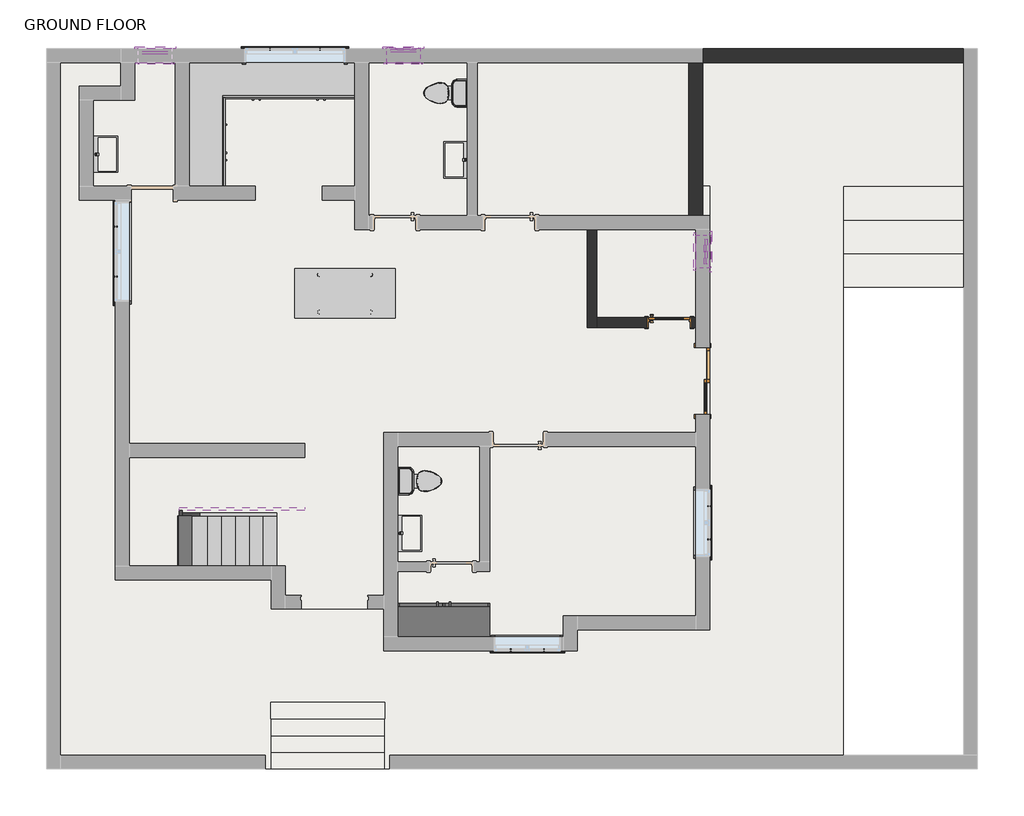
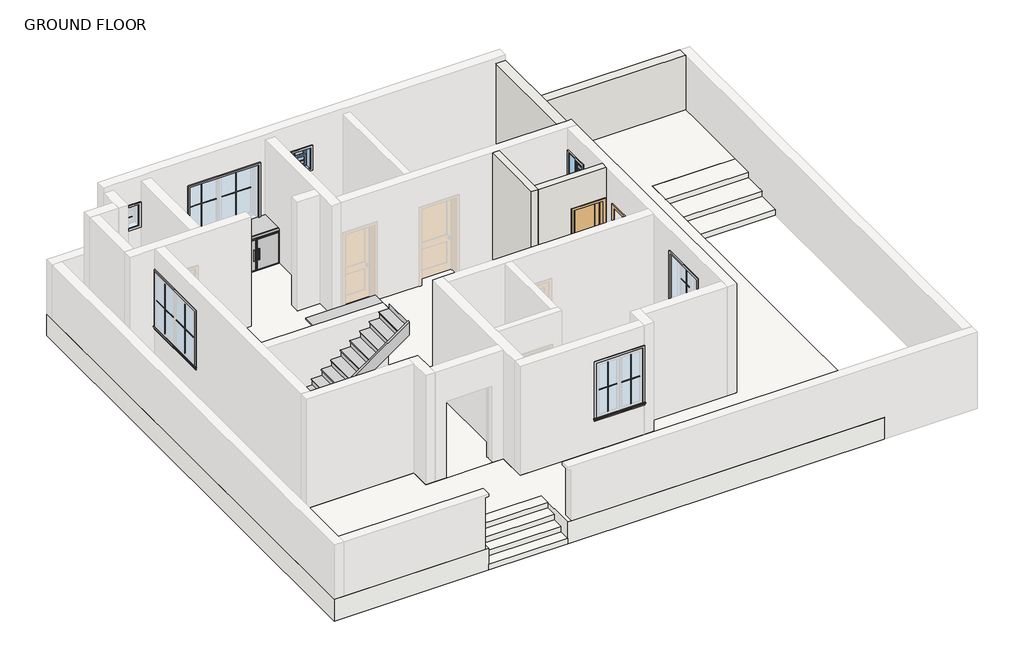
# One storey, part 2 of 2: 30 proxies, 9 slabs, 5 flow terminals, 4 walls, 3 members, 2 doors, 2 windows, 1 furniture element, 1 stair flight.
"""IFC4 building model written with IfcOpenShell, lengths in millimetres."""

from ifc_helpers import new_model, si_unit, frame, origin, origin_with_axes, place, context, project, spatial, polyline, outline, extrude, faceted_brep, transform, mapped, element, save
from components import generic_models_1_generic_models_1_c6f2978c, generic_models_2_generic_models_2_74e35ba5, muntin_pattern_2x2_muntin_pattern_2x2_e751b040, muntin_pattern_2x2_muntin_pattern_2x2_9cc8fee8, muntin_pattern_2x2_muntin_pattern_2x2_6dad3731, muntin_pattern_2x2_muntin_pattern_2x2_a30a3345, muntin_pattern_2x2_muntin_pattern_2x2_cfeb24ad, trim_window_exterior_flat_with_sill_c22f0c79, trim_window_exterior_flat_with_sill_92b9b949, trim_window_exterior_flat_with_sill_858dc10d, trim_window_interior_flat_picture_frame_d1f4d6ef, trim_window_interior_flat_picture_frame_3bb882cf, trim_window_interior_flat_picture_frame_3927330c, door_ae87caab, door_ff2e0a99, toilet_domestic_3d_toilet_domestic_3d_ba6479b0, toilet_domestic_3d_toilet_domestic_3d_30431060, sink_1_0003_sink_1_0003_9aba45dc, new_table_new_table_faa1bdb5, stair_flight_30e1afdc, window_double_hung_2_d0105baa

model = new_model("IFC4")

# Units and contexts
model_context = context("Model", 3, world=origin())
ifc_project = project(units=[si_unit("LENGTHUNIT", "METRE", prefix="MILLI")], contexts=[model_context])

# Site, building, storey
site = spatial("IfcSite", under=ifc_project)
building = spatial("IfcBuilding", under=site)
storey = spatial("IfcBuildingStorey", under=building, Name="GROUND FLOOR", Elevation=0.0)

# Proxies
placement = place(None, origin())
generic_models_1_generic_models_1_shape = generic_models_1_generic_models_1_c6f2978c(model_context)
element("IfcBuildingElementProxy", 1, Name="Generic Models 1 : Generic Models 1", ObjectType="Generic Models 1 : Generic Models 1", at=placement, inside=storey, context=model_context, shape_type="MappedRepresentation", body=[
    mapped(generic_models_1_generic_models_1_shape, transform((0.0, 0.0, 0.0), x_axis=(1.0, 0.0, 0.0), y_axis=(0.0, 1.0, 0.0), z_axis=(0.0, 0.0, 1.0))),
])
generic_models_2_generic_models_2_shape = generic_models_2_generic_models_2_74e35ba5(model_context)
element("IfcBuildingElementProxy", 2, Name="Generic Models 2 : Generic Models 2", ObjectType="Generic Models 2 : Generic Models 2", at=placement, inside=storey, context=model_context, shape_type="MappedRepresentation", body=[
    mapped(generic_models_2_generic_models_2_shape, transform((0.0, 0.0, 0.0), x_axis=(1.0, 0.0, 0.0), y_axis=(0.0, 1.0, 0.0), z_axis=(0.0, 0.0, 1.0))),
])
muntin_pattern_2x2_muntin_pattern_2x2_shape = muntin_pattern_2x2_muntin_pattern_2x2_e751b040(model_context)
element("IfcBuildingElementProxy", 3, Name="Muntin Pattern_2x2 : Muntin Pattern_2x2", ObjectType="Muntin Pattern_2x2 : Muntin Pattern_2x2", at=placement, inside=storey, context=model_context, shape_type="MappedRepresentation", body=[
    mapped(muntin_pattern_2x2_muntin_pattern_2x2_shape, transform((-8676.6951068, 1938.7752014, 984.25), x_axis=(0.0, 1.0, 0.0), y_axis=(-1.0, 0.0, 0.0), z_axis=(0.0, 0.0, 1.0))),
])
element("IfcBuildingElementProxy", 4, Name="Muntin Pattern_2x2 : Muntin Pattern_2x2", ObjectType="Muntin Pattern_2x2 : Muntin Pattern_2x2", at=placement, inside=storey, context=model_context, shape_type="MappedRepresentation", body=[
    mapped(muntin_pattern_2x2_muntin_pattern_2x2_shape, transform((-5865.2326068, 6093.2627014, 984.25), x_axis=(1.0, 0.0, 0.0), y_axis=(0.0, 1.0, 0.0), z_axis=(0.0, 0.0, 1.0))),
])
muntin_pattern_2x2_muntin_pattern_2x2_2_shape = muntin_pattern_2x2_muntin_pattern_2x2_9cc8fee8(model_context)
element("IfcBuildingElementProxy", 5, Name="Muntin Pattern_2x2 : Muntin Pattern_2x2", ObjectType="Muntin Pattern_2x2 : Muntin Pattern_2x2", at=placement, inside=storey, context=model_context, shape_type="MappedRepresentation", body=[
    mapped(muntin_pattern_2x2_muntin_pattern_2x2_2_shape, transform((-8676.6951068, 2850.0002014, 984.25), x_axis=(0.0, -1.0, 0.0), y_axis=(1.0, 0.0, 0.0), z_axis=(0.0, 0.0, 1.0))),
])
element("IfcBuildingElementProxy", 6, Name="Muntin Pattern_2x2 : Muntin Pattern_2x2", ObjectType="Muntin Pattern_2x2 : Muntin Pattern_2x2", at=placement, inside=storey, context=model_context, shape_type="MappedRepresentation", body=[
    mapped(muntin_pattern_2x2_muntin_pattern_2x2_2_shape, transform((-4954.0076068, 6093.2627014, 984.25), x_axis=(-1.0, 0.0, 0.0), y_axis=(0.0, -1.0, 0.0), z_axis=(0.0, 0.0, 1.0))),
])
muntin_pattern_2x2_muntin_pattern_2x2_3_shape = muntin_pattern_2x2_muntin_pattern_2x2_6dad3731(model_context)
element("IfcBuildingElementProxy", 7, Name="Muntin Pattern_2x2 : Muntin Pattern_2x2", ObjectType="Muntin Pattern_2x2 : Muntin Pattern_2x2", at=placement, inside=storey, context=model_context, shape_type="MappedRepresentation", body=[
    mapped(muntin_pattern_2x2_muntin_pattern_2x2_3_shape, transform((-864.6076068, -4885.8872986, 984.25), x_axis=(-1.0, 0.0, 0.0), y_axis=(0.0, -1.0, 0.0), z_axis=(0.0, 0.0, 1.0))),
])
element("IfcBuildingElementProxy", 8, Name="Muntin Pattern_2x2 : Muntin Pattern_2x2", ObjectType="Muntin Pattern_2x2 : Muntin Pattern_2x2", at=placement, inside=storey, context=model_context, shape_type="MappedRepresentation", body=[
    mapped(muntin_pattern_2x2_muntin_pattern_2x2_3_shape, transform((2150.0548932, -2255.3997986, 984.25), x_axis=(0.0, -1.0, 0.0), y_axis=(1.0, 0.0, 0.0), z_axis=(0.0, 0.0, 1.0))),
])
muntin_pattern_2x2_muntin_pattern_2x2_4_shape = muntin_pattern_2x2_muntin_pattern_2x2_a30a3345(model_context)
element("IfcBuildingElementProxy", 9, Name="Muntin Pattern_2x2 : Muntin Pattern_2x2", ObjectType="Muntin Pattern_2x2 : Muntin Pattern_2x2", at=placement, inside=storey, context=model_context, shape_type="MappedRepresentation", body=[
    mapped(muntin_pattern_2x2_muntin_pattern_2x2_4_shape, transform((-1471.0326068, -4885.8872986, 984.25), x_axis=(1.0, 0.0, 0.0), y_axis=(0.0, 1.0, 0.0), z_axis=(0.0, 0.0, 1.0))),
])
element("IfcBuildingElementProxy", 10, Name="Muntin Pattern_2x2 : Muntin Pattern_2x2", ObjectType="Muntin Pattern_2x2 : Muntin Pattern_2x2", at=placement, inside=storey, context=model_context, shape_type="MappedRepresentation", body=[
    mapped(muntin_pattern_2x2_muntin_pattern_2x2_4_shape, transform((2150.0548932, -2861.8247986, 984.25), x_axis=(0.0, 1.0, 0.0), y_axis=(-1.0, 0.0, 0.0), z_axis=(0.0, 0.0, 1.0))),
])
muntin_pattern_2x2_muntin_pattern_2x2_5_shape = muntin_pattern_2x2_muntin_pattern_2x2_cfeb24ad(model_context)
element("IfcBuildingElementProxy", 11, Name="Muntin Pattern_2x2 : Muntin Pattern_2x2", ObjectType="Muntin Pattern_2x2 : Muntin Pattern_2x2", at=placement, inside=storey, context=model_context, shape_type="MappedRepresentation", body=[
    mapped(muntin_pattern_2x2_muntin_pattern_2x2_5_shape, transform((2124.6548932, 2394.3877014, 2155.825), x_axis=(0.0, -1.0, 0.0), y_axis=(1.0, 0.0, 0.0), z_axis=(0.0, 0.0, 1.0))),
])
element("IfcBuildingElementProxy", 12, Name="Muntin Pattern_2x2 : Muntin Pattern_2x2", ObjectType="Muntin Pattern_2x2 : Muntin Pattern_2x2", at=placement, inside=storey, context=model_context, shape_type="MappedRepresentation", body=[
    mapped(muntin_pattern_2x2_muntin_pattern_2x2_5_shape, transform((2080.2048932, 2394.3877014, 1905.0), x_axis=(0.0, -1.0, 0.0), y_axis=(1.0, 0.0, 0.0), z_axis=(0.0, 0.0, 1.0))),
])
element("IfcBuildingElementProxy", 13, Name="Muntin Pattern_2x2 : Muntin Pattern_2x2", ObjectType="Muntin Pattern_2x2 : Muntin Pattern_2x2", at=placement, inside=storey, context=model_context, shape_type="MappedRepresentation", body=[
    mapped(muntin_pattern_2x2_muntin_pattern_2x2_5_shape, transform((-3428.4201068, 6067.8627014, 2155.825), x_axis=(1.0, 0.0, 0.0), y_axis=(0.0, 1.0, 0.0), z_axis=(0.0, 0.0, 1.0))),
])
element("IfcBuildingElementProxy", 14, Name="Muntin Pattern_2x2 : Muntin Pattern_2x2", ObjectType="Muntin Pattern_2x2 : Muntin Pattern_2x2", at=placement, inside=storey, context=model_context, shape_type="MappedRepresentation", body=[
    mapped(muntin_pattern_2x2_muntin_pattern_2x2_5_shape, transform((-3428.4201068, 6023.4127014, 1905.0), x_axis=(1.0, 0.0, 0.0), y_axis=(0.0, 1.0, 0.0), z_axis=(0.0, 0.0, 1.0))),
])
element("IfcBuildingElementProxy", 15, Name="Muntin Pattern_2x2 : Muntin Pattern_2x2", ObjectType="Muntin Pattern_2x2 : Muntin Pattern_2x2", at=placement, inside=storey, context=model_context, shape_type="MappedRepresentation", body=[
    mapped(muntin_pattern_2x2_muntin_pattern_2x2_5_shape, transform((-7962.3201068, 6067.8627014, 2155.825), x_axis=(1.0, 0.0, 0.0), y_axis=(0.0, 1.0, 0.0), z_axis=(0.0, 0.0, 1.0))),
])
element("IfcBuildingElementProxy", 16, Name="Muntin Pattern_2x2 : Muntin Pattern_2x2", ObjectType="Muntin Pattern_2x2 : Muntin Pattern_2x2", at=placement, inside=storey, context=model_context, shape_type="MappedRepresentation", body=[
    mapped(muntin_pattern_2x2_muntin_pattern_2x2_5_shape, transform((-7962.3201068, 6023.4127014, 1905.0), x_axis=(1.0, 0.0, 0.0), y_axis=(0.0, 1.0, 0.0), z_axis=(0.0, 0.0, 1.0))),
])
trim_window_exterior_flat_with_sill_shape = trim_window_exterior_flat_with_sill_c22f0c79(model_context)
element("IfcBuildingElementProxy", 17, Name="Trim-Window-Exterior-Flat : with Sill", ObjectType="Trim-Window-Exterior-Flat : with Sill", at=placement, inside=storey, context=model_context, shape_type="MappedRepresentation", body=[
    mapped(trim_window_exterior_flat_with_sill_shape, transform((-8686.2201068, 2394.3877014, 2438.4), x_axis=(0.0, -1.0, 0.0), y_axis=(0.0, 0.0, 1.0), z_axis=(-1.0, 0.0, 0.0))),
])
element("IfcBuildingElementProxy", 18, Name="Trim-Window-Exterior-Flat : with Sill", ObjectType="Trim-Window-Exterior-Flat : with Sill", at=placement, inside=storey, context=model_context, shape_type="MappedRepresentation", body=[
    mapped(trim_window_exterior_flat_with_sill_shape, transform((-5409.6201068, 6102.7877014, 2438.4), x_axis=(-1.0, 0.0, 0.0), y_axis=(0.0, 0.0, 1.0), z_axis=(0.0, 1.0, 0.0))),
])
trim_window_exterior_flat_with_sill_2_shape = trim_window_exterior_flat_with_sill_92b9b949(model_context)
element("IfcBuildingElementProxy", 19, Name="Trim-Window-Exterior-Flat : with Sill", ObjectType="Trim-Window-Exterior-Flat : with Sill", at=placement, inside=storey, context=model_context, shape_type="MappedRepresentation", body=[
    mapped(trim_window_exterior_flat_with_sill_2_shape, transform((-1167.8201068, -4895.4122986, 2438.4), x_axis=(1.0, 0.0, 0.0), y_axis=(0.0, 0.0, 1.0), z_axis=(0.0, -1.0, 0.0))),
])
element("IfcBuildingElementProxy", 20, Name="Trim-Window-Exterior-Flat : with Sill", ObjectType="Trim-Window-Exterior-Flat : with Sill", at=placement, inside=storey, context=model_context, shape_type="MappedRepresentation", body=[
    mapped(trim_window_exterior_flat_with_sill_2_shape, transform((2159.5798932, -2558.6122986, 2438.4), x_axis=(0.0, 1.0, 0.0), y_axis=(0.0, 0.0, 1.0), z_axis=(1.0, 0.0, 0.0))),
])
trim_window_exterior_flat_with_sill_3_shape = trim_window_exterior_flat_with_sill_858dc10d(model_context)
element("IfcBuildingElementProxy", 21, Name="Trim-Window-Exterior-Flat : with Sill", ObjectType="Trim-Window-Exterior-Flat : with Sill", at=placement, inside=storey, context=model_context, shape_type="MappedRepresentation", body=[
    mapped(trim_window_exterior_flat_with_sill_3_shape, transform((2159.5798932, 2394.3877014, 2438.4), x_axis=(0.0, 1.0, 0.0), y_axis=(0.0, 0.0, 1.0), z_axis=(1.0, 0.0, 0.0))),
])
element("IfcBuildingElementProxy", 22, Name="Trim-Window-Exterior-Flat : with Sill", ObjectType="Trim-Window-Exterior-Flat : with Sill", at=placement, inside=storey, context=model_context, shape_type="MappedRepresentation", body=[
    mapped(trim_window_exterior_flat_with_sill_3_shape, transform((-3428.4201068, 6102.7877014, 2438.4), x_axis=(-1.0, 0.0, 0.0), y_axis=(0.0, 0.0, 1.0), z_axis=(0.0, 1.0, 0.0))),
])
element("IfcBuildingElementProxy", 23, Name="Trim-Window-Exterior-Flat : with Sill", ObjectType="Trim-Window-Exterior-Flat : with Sill", at=placement, inside=storey, context=model_context, shape_type="MappedRepresentation", body=[
    mapped(trim_window_exterior_flat_with_sill_3_shape, transform((-7962.3201068, 6102.7877014, 2438.4), x_axis=(-1.0, 0.0, 0.0), y_axis=(0.0, 0.0, 1.0), z_axis=(0.0, 1.0, 0.0))),
])
trim_window_interior_flat_picture_frame_shape = trim_window_interior_flat_picture_frame_d1f4d6ef(model_context)
element("IfcBuildingElementProxy", 24, Name="Trim-Window-Interior-Flat : Picture Frame", ObjectType="Trim-Window-Interior-Flat : Picture Frame", at=placement, inside=storey, context=model_context, shape_type="MappedRepresentation", body=[
    mapped(trim_window_interior_flat_picture_frame_shape, transform((-8432.2201068, 2394.3877014, 2438.4), x_axis=(0.0, 1.0, 0.0), y_axis=(0.0, 0.0, 1.0), z_axis=(1.0, 0.0, 0.0))),
])
element("IfcBuildingElementProxy", 25, Name="Trim-Window-Interior-Flat : Picture Frame", ObjectType="Trim-Window-Interior-Flat : Picture Frame", at=placement, inside=storey, context=model_context, shape_type="MappedRepresentation", body=[
    mapped(trim_window_interior_flat_picture_frame_shape, transform((-5409.6201068, 5848.7877014, 2438.4), x_axis=(1.0, 0.0, 0.0), y_axis=(0.0, 0.0, 1.0), z_axis=(0.0, -1.0, 0.0))),
])
trim_window_interior_flat_picture_frame_2_shape = trim_window_interior_flat_picture_frame_3bb882cf(model_context)
element("IfcBuildingElementProxy", 26, Name="Trim-Window-Interior-Flat : Picture Frame", ObjectType="Trim-Window-Interior-Flat : Picture Frame", at=placement, inside=storey, context=model_context, shape_type="MappedRepresentation", body=[
    mapped(trim_window_interior_flat_picture_frame_2_shape, transform((-1167.8201068, -4641.4122986, 2438.4), x_axis=(-1.0, 0.0, 0.0), y_axis=(0.0, 0.0, 1.0), z_axis=(0.0, 1.0, 0.0))),
])
element("IfcBuildingElementProxy", 27, Name="Trim-Window-Interior-Flat : Picture Frame", ObjectType="Trim-Window-Interior-Flat : Picture Frame", at=placement, inside=storey, context=model_context, shape_type="MappedRepresentation", body=[
    mapped(trim_window_interior_flat_picture_frame_2_shape, transform((1905.5798932, -2558.6122986, 2438.4), x_axis=(0.0, -1.0, 0.0), y_axis=(0.0, 0.0, 1.0), z_axis=(-1.0, 0.0, 0.0))),
])
trim_window_interior_flat_picture_frame_3_shape = trim_window_interior_flat_picture_frame_3927330c(model_context)
element("IfcBuildingElementProxy", 28, Name="Trim-Window-Interior-Flat : Picture Frame", ObjectType="Trim-Window-Interior-Flat : Picture Frame", at=placement, inside=storey, context=model_context, shape_type="MappedRepresentation", body=[
    mapped(trim_window_interior_flat_picture_frame_3_shape, transform((1905.5798932, 2394.3877014, 2438.4), x_axis=(0.0, -1.0, 0.0), y_axis=(0.0, 0.0, 1.0), z_axis=(-1.0, 0.0, 0.0))),
])
element("IfcBuildingElementProxy", 29, Name="Trim-Window-Interior-Flat : Picture Frame", ObjectType="Trim-Window-Interior-Flat : Picture Frame", at=placement, inside=storey, context=model_context, shape_type="MappedRepresentation", body=[
    mapped(trim_window_interior_flat_picture_frame_3_shape, transform((-3428.4201068, 5848.7877014, 2438.4), x_axis=(1.0, 0.0, 0.0), y_axis=(0.0, 0.0, 1.0), z_axis=(0.0, -1.0, 0.0))),
])
element("IfcBuildingElementProxy", 30, Name="Trim-Window-Interior-Flat : Picture Frame", ObjectType="Trim-Window-Interior-Flat : Picture Frame", at=placement, inside=storey, context=model_context, shape_type="MappedRepresentation", body=[
    mapped(trim_window_interior_flat_picture_frame_3_shape, transform((-7962.3201068, 5848.7877014, 2438.4), x_axis=(1.0, 0.0, 0.0), y_axis=(0.0, 0.0, 1.0), z_axis=(0.0, -1.0, 0.0))),
])

# Doors
door_shape = door_ae87caab(model_context)
element("IfcDoor", 31, ObjectType="Door-Double-Sliding : 48\" x 84\"", at=placement, inside=storey, context=model_context, shape_type="MappedRepresentation", body=[
    mapped(door_shape, transform((1905.5798932, 32.1877014, 0.0), x_axis=(0.0, -1.0, 0.0), y_axis=(1.0, 0.0, 0.0), z_axis=(0.0, 0.0, 1.0))),
])
door_2_shape = door_ff2e0a99(model_context)
element("IfcDoor", 32, ObjectType="Door-Interior-Single-2_Panel-Wood : 2'6\"", at=placement, inside=storey, context=model_context, shape_type="MappedRepresentation", body=[
    mapped(door_2_shape, transform((1422.9798932, 1102.1627014, 0.0), x_axis=(1.0, 0.0, 0.0), y_axis=(0.0, 1.0, 0.0), z_axis=(0.0, 0.0, 1.0))),
])

# Flow terminals
toilet_domestic_3d_toilet_domestic_3d_shape = toilet_domestic_3d_toilet_domestic_3d_ba6479b0(model_context)
toilet_domestic_3d_toilet_domestic_3d_2_shape = toilet_domestic_3d_toilet_domestic_3d_30431060(model_context)
element("IfcFlowTerminal", 33, ObjectType="Toilet-Domestic-3D : Toilet-Domestic-3D", at=placement, inside=storey, context=model_context, shape_type="MappedRepresentation", body=[
    mapped(toilet_domestic_3d_toilet_domestic_3d_shape, transform((-3035.3240795, -1796.6122986, 0.0), x_axis=(0.0, 1.0, 0.0), y_axis=(-1.0, 0.0, 0.0), z_axis=(0.0, 0.0, 1.0))),
    mapped(toilet_domestic_3d_toilet_domestic_3d_2_shape, transform((-3035.3240795, -1796.6122986, 0.0), x_axis=(0.0, 1.0, 0.0), y_axis=(-1.0, 0.0, 0.0), z_axis=(0.0, 0.0, 1.0))),
])
element("IfcFlowTerminal", 34, ObjectType="Toilet-Domestic-3D : Toilet-Domestic-3D", at=placement, inside=storey, context=model_context, shape_type="MappedRepresentation", body=[
    mapped(toilet_domestic_3d_toilet_domestic_3d_shape, transform((-2754.7161342, 5289.9877014, 0.0), x_axis=(0.0, -1.0, 0.0), y_axis=(1.0, 0.0, 0.0), z_axis=(0.0, 0.0, 1.0))),
    mapped(toilet_domestic_3d_toilet_domestic_3d_2_shape, transform((-2754.7161342, 5289.9877014, 0.0), x_axis=(0.0, -1.0, 0.0), y_axis=(1.0, 0.0, 0.0), z_axis=(0.0, 0.0, 1.0))),
])
sink_1_0003_sink_1_0003_shape = sink_1_0003_sink_1_0003_9aba45dc(model_context)
element("IfcFlowTerminal", 35, ObjectType="sink 1.0003 : sink 1.0003", at=placement, inside=storey, context=model_context, shape_type="MappedRepresentation", body=[
    mapped(sink_1_0003_sink_1_0003_shape, transform((-2475.9201068, 4070.7877014, 0.0), x_axis=(1.0, 0.0, 0.0), y_axis=(0.0, 1.0, 0.0), z_axis=(0.0, 0.0, 1.0))),
])
element("IfcFlowTerminal", 36, ObjectType="sink 1.0003 : sink 1.0003", at=placement, inside=storey, context=model_context, shape_type="MappedRepresentation", body=[
    mapped(sink_1_0003_sink_1_0003_shape, transform((-8864.0201068, 4172.3877014, 0.0), x_axis=(-1.0, 0.0, 0.0), y_axis=(0.0, -1.0, 0.0), z_axis=(0.0, 0.0, 1.0))),
])
element("IfcFlowTerminal", 37, ObjectType="sink 1.0003 : sink 1.0003", at=placement, inside=storey, context=model_context, shape_type="MappedRepresentation", body=[
    mapped(sink_1_0003_sink_1_0003_shape, transform((-3314.1201068, -2749.1122986, 0.0), x_axis=(-1.0, 0.0, 0.0), y_axis=(0.0, -1.0, 0.0), z_axis=(0.0, 0.0, 1.0))),
])

# Furniture
new_table_new_table_shape = new_table_new_table_faa1bdb5(model_context)
element("IfcFurniture", 38, ObjectType="new table : new table", at=placement, inside=storey, context=model_context, shape_type="MappedRepresentation", body=[
    mapped(new_table_new_table_shape, transform((-4495.2201068, 1632.3877014, 0.0), x_axis=(1.0, 0.0, 0.0), y_axis=(0.0, 1.0, 0.0), z_axis=(0.0, 0.0, 1.0))),
])

# Members
element("IfcMember", 39, ObjectType="Stringer - 2\" Width", at=placement, inside=storey, context=model_context, shape_type="SweptSolid", body=[
    extrude(outline(polyline([(0.0, -5739.8201068), (221.519187, -5739.8201068), (1430.559187, -7467.0201068), (1058.5033718, -7467.0201068), (0.0, -5954.8724328), (0.0, -5739.8201068)])), frame((0.0, -2431.6122986, 0.0), z_axis=(0.0, 1.0, 0.0), x_axis=(0.0, 0.0, 1.0)), (0.0, 0.0, 1.0), 50.8),
])
element("IfcMember", 40, ObjectType="Stringer - 2\" Width", at=placement, inside=storey, context=model_context, shape_type="SweptSolid", body=[
    extrude(outline(polyline([(-7467.0201068, -2431.6122986), (-7517.8201068, -2431.6122986), (-7517.8201068, -2330.0122986), (-7467.0201068, -2330.0122986), (-7467.0201068, -2431.6122986)])), frame((0.0, 0.0, 1193.8), z_axis=(0.0, 0.0, 1.0), x_axis=(1.0, 0.0, 0.0)), (0.0, 0.0, 1.0), 304.8),
])
element("IfcMember", 41, ObjectType="Stringer - 2\" Width", at=placement, inside=storey, context=model_context, shape_type="SweptSolid", body=[
    extrude(outline(polyline([(1643.919187, -7517.8201068), (1271.8633718, -7517.8201068), (2872.0633718, -5231.8201068), (3244.119187, -5231.8201068), (1643.919187, -7517.8201068)])), frame((0.0, -2330.0122986, 0.0), z_axis=(0.0, 1.0, 0.0), x_axis=(0.0, 0.0, 1.0)), (0.0, 0.0, 1.0), 50.8),
])

# Slabs
element("IfcSlab", 42, ObjectType="2'", at=placement, inside=storey, context=model_context, shape_type="Brep", body=[
    faceted_brep([(2032.5798932, 6102.7877014, -609.6), (7049.0798932, 6102.7877014, -609.6), (7049.0798932, 3588.1877014, -609.6), (4597.9798932, 3588.1877014, -609.6), (4597.9798932, -6800.4122986, -609.6), (4597.9798932, -7054.4122986, -609.6), (-3771.3201068, -7054.4122986, -609.6), (-3771.3201068, -5835.2122986, -609.6), (-5854.1201068, -5835.2122986, -609.6), (-5854.1201068, -7054.4122986, -609.6), (-9943.5201068, -7054.4122986, -609.6), (-9943.5201068, 6102.7877014, -609.6), (-5841.4201068, -3600.0122986, -609.6), (-5841.4201068, -4133.4122986, -609.6), (-3784.0201068, -4133.4122986, -609.6), (-3784.0201068, -4895.4122986, -609.6), (-253.4201068, -4895.4122986, -609.6), (-253.4201068, -4514.4122986, -609.6), (2159.5798932, -4514.4122986, -609.6), (2159.5798932, 3588.1877014, -609.6), (2032.5798932, 3588.1877014, -609.6), (2032.5798932, 5848.7877014, -609.6), (-8584.6201068, 5848.7877014, -609.6), (-8584.6201068, 5416.9877014, -609.6), (-9346.6201068, 5416.9877014, -609.6), (-9346.6201068, 3334.1877014, -609.6), (-8686.2201068, 3334.1877014, -609.6), (-8686.2201068, -3600.0122986, -609.6), (2032.5798932, 6102.7877014, 0.0), (-9943.5201068, 6102.7877014, 0.0), (-9943.5201068, -7054.4122986, 0.0), (-9689.5201068, -7054.4122986, 0.0), (-5948.2201068, -7054.4122986, 0.0), (-5854.1201068, -7054.4122986, 0.0), (-5854.1201068, -5835.2122986, 0.0), (-3771.3201068, -5835.2122986, 0.0), (-3771.3201068, -7054.4122986, 0.0), (-3677.2201068, -7054.4122986, 0.0), (4597.9798932, -7054.4122986, 0.0), (4597.9798932, -6800.4122986, 0.0), (4597.9798932, 3588.1877014, 0.0), (7049.0798932, 3588.1877014, 0.0), (7049.0798932, 6102.7877014, 0.0), (6795.0798932, 6102.7877014, 0.0), (-5841.4201068, -3600.0122986, 0.0), (-8686.2201068, -3600.0122986, 0.0), (-8686.2201068, 3334.1877014, 0.0), (-9346.6201068, 3334.1877014, 0.0), (-9346.6201068, 5416.9877014, 0.0), (-8584.6201068, 5416.9877014, 0.0), (-8584.6201068, 5848.7877014, 0.0), (2032.5798932, 5848.7877014, 0.0), (2032.5798932, 3588.1877014, 0.0), (2159.5798932, 3588.1877014, 0.0), (2159.5798932, -4514.4122986, 0.0), (-253.4201068, -4514.4122986, 0.0), (-253.4201068, -4895.4122986, 0.0), (-3784.0201068, -4895.4122986, 0.0), (-3784.0201068, -4133.4122986, 0.0), (-5841.4201068, -4133.4122986, 0.0)], [[[0, 1, 2, 3, 4, 5, 6, 7, 8, 9, 10, 11], [12, 13, 14, 15, 16, 17, 18, 19, 20, 21, 22, 23, 24, 25, 26, 27]], [[28, 29, 30, 31, 32, 33, 34, 35, 36, 37, 38, 39, 40, 41, 42, 43], [44, 45, 46, 47, 48, 49, 50, 51, 52, 53, 54, 55, 56, 57, 58, 59]], [[5, 4, 3, 40, 39, 38]], [[6, 5, 38, 37, 36]], [[11, 10, 30, 29]], [[0, 11, 29, 28]], [[1, 0, 28, 43, 42]], [[2, 1, 42, 41]], [[3, 2, 41, 40]], [[13, 12, 44, 59]], [[14, 13, 59, 58]], [[15, 14, 58, 57]], [[16, 15, 57, 56]], [[17, 16, 56, 55]], [[18, 17, 55, 54]], [[19, 18, 54, 53]], [[20, 19, 53, 52]], [[21, 20, 52, 51]], [[22, 21, 51, 50]], [[23, 22, 50, 49]], [[24, 23, 49, 48]], [[25, 24, 48, 47]], [[26, 25, 47, 46]], [[27, 26, 46, 45]], [[12, 27, 45, 44]], [[7, 6, 36, 35]], [[8, 7, 35, 34]], [[9, 8, 34, 33]], [[10, 9, 33, 32, 31, 30]]]),
])
element("IfcSlab", 43, ObjectType="2' 2", at=placement, inside=storey, context=model_context, shape_type="SweptSolid", body=[
    extrude(outline(polyline([(2032.5798932, 5848.7877014), (2032.5798932, 3588.1877014), (2159.5798932, 3588.1877014), (2159.5798932, -4514.4122986), (-253.4201068, -4514.4122986), (-253.4201068, -4895.4122986), (-3784.0201068, -4895.4122986), (-3784.0201068, -4133.4122986), (-5841.4201068, -4133.4122986), (-5841.4201068, -3600.0122986), (-8686.2201068, -3600.0122986), (-8686.2201068, 3334.1877014), (-9346.6201068, 3334.1877014), (-9346.6201068, 5416.9877014), (-8584.6201068, 5416.9877014), (-8584.6201068, 5848.7877014), (2032.5798932, 5848.7877014)])), frame((0.0, 0.0, -609.6), z_axis=(0.0, 0.0, 1.0), x_axis=(1.0, 0.0, 0.0)), (0.0, 0.0, 1.0), 609.6),
])
element("IfcSlab", 44, ObjectType="2' 5", at=placement, inside=storey, context=model_context, shape_type="SweptSolid", body=[
    extrude(outline(polyline([(-3771.3201068, -5835.2122986), (-3771.3201068, -7054.4122986), (-5854.1201068, -7054.4122986), (-5854.1201068, -5835.2122986), (-3771.3201068, -5835.2122986)])), frame((0.0, 0.0, -609.6), z_axis=(0.0, 0.0, 1.0), x_axis=(1.0, 0.0, 0.0)), (0.0, 0.0, 1.0), 152.4),
])
element("IfcSlab", 45, ObjectType="2' 5", at=placement, inside=storey, context=model_context, shape_type="SweptSolid", body=[
    extrude(outline(polyline([(-3771.3201068, -5835.2122986), (-3771.3201068, -6749.6122986), (-5854.1201068, -6749.6122986), (-5854.1201068, -5835.2122986), (-3771.3201068, -5835.2122986)])), frame((0.0, 0.0, -457.2), z_axis=(0.0, 0.0, 1.0), x_axis=(1.0, 0.0, 0.0)), (0.0, 0.0, 1.0), 152.4),
])
element("IfcSlab", 46, ObjectType="2' 5", at=placement, inside=storey, context=model_context, shape_type="SweptSolid", body=[
    extrude(outline(polyline([(-3771.3201068, -5835.2122986), (-3771.3201068, -6444.8122986), (-5854.1201068, -6444.8122986), (-5854.1201068, -5835.2122986), (-3771.3201068, -5835.2122986)])), frame((0.0, 0.0, -304.8), z_axis=(0.0, 0.0, 1.0), x_axis=(1.0, 0.0, 0.0)), (0.0, 0.0, 1.0), 152.4),
])
element("IfcSlab", 47, ObjectType="2' 5", at=placement, inside=storey, context=model_context, shape_type="SweptSolid", body=[
    extrude(outline(polyline([(-3771.3201068, -5835.2122986), (-3771.3201068, -6140.0122986), (-5854.1201068, -6140.0122986), (-5854.1201068, -5835.2122986), (-3771.3201068, -5835.2122986)])), frame((0.0, 0.0, -152.4), z_axis=(0.0, 0.0, 1.0), x_axis=(1.0, 0.0, 0.0)), (0.0, 0.0, 1.0), 152.4),
])
element("IfcSlab", 48, ObjectType="6\"", at=placement, inside=storey, context=model_context, shape_type="Brep", body=[
    faceted_brep([(7049.0798932, 3588.1877014, -457.2), (7049.0798932, 1746.6877014, -457.2), (6795.0798932, 1746.6877014, -457.2), (4597.9798932, 1746.6877014, -457.2), (4597.9798932, 3588.1877014, -457.2), (7049.0798932, 3588.1877014, -304.8), (4597.9798932, 3588.1877014, -304.8), (4597.9798932, 1746.6877014, -304.8), (6795.0798932, 1746.6877014, -304.8), (7049.0798932, 1746.6877014, -304.8), (7049.0798932, 2356.2877014, -304.8)], [[[0, 1, 2, 3, 4]], [[5, 6, 7, 8, 9, 10]], [[1, 0, 5, 10, 9]], [[3, 2, 1, 9, 8, 7]], [[4, 3, 7, 6]], [[0, 4, 6, 5]]]),
])
element("IfcSlab", 49, ObjectType="6\"", at=placement, inside=storey, context=model_context, shape_type="Brep", body=[
    faceted_brep([(7049.0798932, 3588.1877014, -304.8), (7049.0798932, 2356.2877014, -304.8), (6795.0798932, 2356.2877014, -304.8), (4597.9798932, 2356.2877014, -304.8), (4597.9798932, 3588.1877014, -304.8), (7049.0798932, 3588.1877014, -152.4), (4597.9798932, 3588.1877014, -152.4), (4597.9798932, 2356.2877014, -152.4), (6795.0798932, 2356.2877014, -152.4), (7049.0798932, 2356.2877014, -152.4), (7049.0798932, 2972.2377014, -152.4)], [[[0, 1, 2, 3, 4]], [[5, 6, 7, 8, 9, 10]], [[1, 0, 5, 10, 9]], [[3, 2, 1, 9, 8, 7]], [[4, 3, 7, 6]], [[0, 4, 6, 5]]]),
])
element("IfcSlab", 50, ObjectType="6\"", at=placement, inside=storey, context=model_context, shape_type="Brep", body=[
    faceted_brep([(7049.0798932, 3588.1877014, -152.4), (7049.0798932, 2972.2377014, -152.4), (6795.0798932, 2972.2377014, -152.4), (4597.9798932, 2972.2377014, -152.4), (4597.9798932, 3588.1877014, -152.4), (7049.0798932, 3588.1877014, 0.0), (4597.9798932, 3588.1877014, 0.0), (4597.9798932, 2972.2377014, 0.0), (6795.0798932, 2972.2377014, 0.0), (7049.0798932, 2972.2377014, 0.0)], [[[0, 1, 2, 3, 4]], [[5, 6, 7, 8, 9]], [[1, 0, 5, 9]], [[3, 2, 1, 9, 8, 7]], [[4, 3, 7, 6]], [[0, 4, 6, 5]]]),
])

# Stair flight
stair_flight_shape = stair_flight_30e1afdc(model_context)
element("IfcStairFlight", 51, ObjectType="2\" Tread 1\" Nosing 1/4\" Riser", at=placement, inside=storey, context=model_context, shape_type="MappedRepresentation", body=[
    mapped(stair_flight_shape, transform((0.0, 0.0, 0.0), x_axis=(1.0, 0.0, 0.0), y_axis=(0.0, 1.0, 0.0), z_axis=(0.0, 0.0, 1.0))),
])

# Walls
element("IfcWall", 52, at=placement, inside=storey, context=model_context, shape_type="Brep", body=[
    faceted_brep([(1778.5798932, 5848.7877014, 0.0), (1778.5798932, 3054.7877014, 0.0), (1778.5798932, 3054.7877014, 3048.0), (1778.5798932, 5848.7877014, 3048.0), (2032.5798932, 3054.7877014, 0.0), (2032.5798932, 5848.7877014, 0.0), (2032.5798932, 5848.7877014, 3048.0), (2032.5798932, 3588.1877014, 3048.0), (2032.5798932, 3054.7877014, 3048.0)], [[[0, 1, 2, 3]], [[4, 5, 6, 7, 8]], [[1, 0, 5, 4]], [[1, 4, 8, 2]], [[5, 0, 3, 6]], [[3, 2, 8, 7, 6]]]),
])
element("IfcWall", 53, at=placement, inside=storey, context=model_context, shape_type="SweptSolid", body=[
    extrude(outline(polyline([(2032.5798932, 6102.7877014), (6795.0798932, 6102.7877014), (6795.0798932, 5848.7877014), (2032.5798932, 5848.7877014), (2032.5798932, 6102.7877014)])), origin_with_axes(), (0.0, 0.0, 1.0), 1524.0),
])
element("IfcWall", 54, ObjectType="6\" WALL", at=placement, inside=storey, context=model_context, shape_type="Brep", body=[
    faceted_brep([(-75.6201068, 2800.7877014, 0.0), (-75.6201068, 1010.0877014, 0.0), (-75.6201068, 1010.0877014, 3048.0), (-75.6201068, 2800.7877014, 3048.0), (102.1798932, 1010.0877014, 0.0), (102.1798932, 1187.8877014, 0.0), (102.1798932, 2800.7877014, 0.0), (102.1798932, 2800.7877014, 3048.0), (102.1798932, 1187.8877014, 3048.0), (102.1798932, 1010.0877014, 3048.0)], [[[0, 1, 2, 3]], [[4, 5, 6, 7, 8, 9]], [[1, 0, 6, 5, 4]], [[6, 0, 3, 7]], [[1, 4, 9, 2]], [[3, 2, 9, 8, 7]]]),
])
element("IfcWall", 55, ObjectType="6\" WALL", at=placement, inside=storey, context=model_context, shape_type="SweptSolid", body=[
    extrude(outline(polyline([(0.0, 1829.3798932), (0.0, 1905.5798932), (3048.0, 1905.5798932), (3048.0, 102.1798932), (0.0, 102.1798932), (0.0, 1016.5798932), (2159.0, 1016.5798932), (2159.0, 1829.3798932), (0.0, 1829.3798932)])), frame((0.0, 1010.0877014, 0.0), z_axis=(0.0, 1.0, 0.0), x_axis=(0.0, 0.0, 1.0)), (0.0, 0.0, 1.0), 177.8),
])

# Windows
window_double_hung_2_shape = window_double_hung_2_d0105baa(model_context)
element("IfcWindow", 56, ObjectType="Window-Double-Hung : 2'", at=placement, inside=storey, context=model_context, shape_type="MappedRepresentation", body=[
    mapped(window_double_hung_2_shape, transform((2032.5798932, 2394.3877014, 914.4), x_axis=(0.0, -1.0, 0.0), y_axis=(1.0, 0.0, 0.0), z_axis=(0.0, 0.0, 1.0))),
])
element("IfcWindow", 57, ObjectType="Window-Double-Hung : 2'", at=placement, inside=storey, context=model_context, shape_type="MappedRepresentation", body=[
    mapped(window_double_hung_2_shape, transform((-3428.4201068, 5975.7877014, 914.4), x_axis=(1.0, 0.0, 0.0), y_axis=(0.0, 1.0, 0.0), z_axis=(0.0, 0.0, 1.0))),
])

save(model, "model.ifc")

# Revit data of these elements
# Type "Muntin Pattern_2x2 : Muntin Pattern_2x2"
#   Width [instance default] = 4' - 0"
#   Thickness = 0' - 0 1/2"
#   Height [instance default] = 4' - 0"
#   Distance = 0' - 0 3/4"
#   Interior Material [instance default] = none
#   Exterior Material [instance default] = none
#   Default Elevation = 0
# Type "Trim-Window-Exterior-Flat : with Sill"
#   Trim Width = 0' - 2 1/4"
#   Trim Thickness_Picture Frame = 0' - 1 1/4"
#   Trim Thickness_with Sill = 0' - 0 3/4"
#   Sill Thickness = 0' - 1 1/4"
#   Opening Width [instance default] = 2' - 0"
#   Opening Height [instance default] = 3' - 0"
#   Default Elevation = 4' - 0"
#   Sill = yes
#   Picture Frame = no
#   Trim Material [instance default] = none
# Type "Trim-Window-Interior-Flat : Picture Frame"
#   Trim Thickness_Picture Frame = 0' - 1 1/4"
#   Trim Width = 0' - 2 1/4"
#   Trim Thickness_with Sill = 0' - 0 3/4"
#   Sill Thickness = 0' - 1 1/4"
#   Opening Width [instance default] = 2' - 0"
#   Opening Height [instance default] = 3' - 0"
#   Default Elevation = 4' - 0"
#   Sill = no
#   Picture Frame = yes
#   Trim Material [instance default] = none
# Type "Door-Double-Sliding : 48\" x 84\""
#   Type Mark = "11"
#   Construction Type Id = "opn-d45"
#   Assembly Code = "C1020"
#   Analytic Construction = "Wood frame, double glass door "
#   Thickness = 0' - 2"
#   Thermal Resistance (R) = 1.8150 (h·ft²·°F)/BTU
#   Heat Transfer Coefficient (U) = 0.5510 BTU/(h·ft²·°F)
#   Height = 7' - 0"
#   Rail Width = 0' - 2"
#   Stiles = 0' - 2"
#   Trim Projection Ext = 0' - 1"
#   Trim Projection Int = 0' - 1"
#   Trim Width = 0' - 3"
#   Width = 4' - 0"
#   Define Thermal Properties by = 1
#   Glazing = Glass
#   Panel Material = Wood - Birch - Solid Stained Light Low Gloss
#   Trim Material = Paint - Sienna
#   Visual Light Transmittance = 0
#   Solar Heat Gain Coefficient = 0
#   Function = (empty or 0)
#   Wall Closure = (empty or 0)
# Type "Door-Interior-Single-2_Panel-Wood : 2'6\""
#   Type Mark = "10"
#   Assembly Code = "C1020300"
#   Analytic Construction = "Wooden"
#   Top Rail = 0' - 4 11/16"
#   Thickness = 0' - 1 3/8"
#   Thermal Resistance (R) = 2.5876 (h·ft²·°F)/BTU
#   Swing Angle [instance default] = 90.00°
#   Stiles = 0' - 4 3/4"
#   Rough Width = 2' - 8"
#   Rough Height = 7' - 1"
#   Lock Rail = 0' - 7 1/2"
#   Height = 7' - 0"
#   Width = 2' - 6"
#   Heat Transfer Coefficient (U) = 0.3865 BTU/(h·ft²·°F)
#   Bottom Rail = 0' - 9 1/8"
#   Trim Material = Cherry
#   Panel Material = Cherry
#   Frame Material = Cherry
#   Door Handle Material = Aluminum
#   Visual Light Transmittance = 0
#   Solar Heat Gain Coefficient = 0
#   Wall Closure = (empty or 0)
#   Function = (empty or 0)
# Type "Toilet-Domestic-3D : Toilet-Domestic-3D"
#   Assembly Code = "D2010110"
#   Toilet - Bowl/Basin Material = Porcelain, Linen
#   Toilet - Seat Material = Laminate, Linen, Matte
#   Default Elevation = 0
# Type "sink 1.0003 : sink 1.0003"
#   Default Elevation = 0
# Type "new table : new table"
#   Default Elevation = 0
# Type "2'"
#   Assembly Code = "B1010"
#   Function = 0
#   Layers, outside or top first: 2' - 0" "Default New Material(1)" (function 1)
# Type "2' 2"
#   Assembly Code = "B1010"
#   Function = 0
#   Layers, outside or top first: 2' - 0" "0 floor" (function 1)
# Type "2' 5"
#   Assembly Code = "B1010"
#   Function = 0
#   Layers, outside or top first: 0' - 6" "Default New Material(1)" (function 1)
# Type "6\""
#   Assembly Code = "B1010"
#   Function = 0
#   Layers, outside or top first: 0' - 6" "0 floor outer" (function 1)
# Type
#   Assembly Code = "B2010"
#   Layers, outside or top first: 0' - 0 1/2" "0 olive green light" (function 4); 0' - 9" no material (function 1); 0' - 0 1/2" "0 olive green light" (function 4)
# Type "6\" WALL"
#   Assembly Code = "B2010"
#   Layers, outside or top first: 0' - 0 1/2" "0 olive green light" (function 4); 0' - 6" no material (function 1); 0' - 0 1/2" "0 olive green light" (function 4)
# Type "Window-Double-Hung : 2'"
#   Type Mark = "20"
#   Fire Rating = "0.5h"
#   Construction Type Id = "DG-DR"
#   Assembly Code = "B2020100"
#   Analytic Construction = "Double glazing - domestic"
#   Wall Thickness [instance default] = 0' - 6"
#   Window Inset [instance default] = 0' - 0"
#   Visual Light Transmittance = 0.81
#   Thermal Resistance (R) = 1.8146 (h·ft²·°F)/BTU
#   Solar Heat Gain Coefficient = 0.76
#   Muntin Width = 1' - 6"
#   Muntin Height = 0' - 8 1/8"
#   Interior Wall Closure [instance default] = 0' - 1 1/2"
#   Rough Width = 2' - 0 1/2"
#   Rough Height = 2' - 0 1/2"
#   Frame Extension [instance default] = 0' - 1 1/4"
#   Exterior Wall Closure [instance default] = 0' - 0 1/2"
#   Extension Jamb [instance default] = 0' - 1 1/2"
#   Heat Transfer Coefficient (U) = 0.5511 BTU/(h·ft²·°F)
#   Height = 2' - 0"
#   Width = 2' - 0"
#   Top Muntin Visibility = yes
#   Indicator Visibility [instance default] = yes
#   Extension Jamb Visibility [instance default] = yes
#   Interior Trim Visibility [instance default] = yes
#   Exterior Trim Visibility [instance default] = yes
#   Define Thermal Properties by = 1
#   Bottom Muntin Visibility = yes
#   Muntin Pattern = Muntin Pattern_2x2 : Muntin Pattern_2x2
#   Interior Trim Material = Wood - Stained
#   Interior Trim = Trim-Window-Interior-Flat : Picture Frame
#   Exterior Trim Material = Clad - White
#   Exterior Trim = Trim-Window-Exterior-Flat : with Sill
#   Glass Panel Material = Glass
#   Exterior Frame Material = Clad - White
#   Interior Frame Material = Wood - Stained
#   Wall Closure = (empty or 0)
# Element 1 (IfcBuildingElementProxy, "Generic Models 1 : Generic Models 1")
#   Phase Created = New Construction
#   Materials on its faces: "0 kitchen tiles(1)", "0 kitchen tiles(2)", "0 kitchen tiles(3)", "0 kitchen tiles"
# Element 2 (IfcBuildingElementProxy, "Generic Models 2 : Generic Models 2")
#   Phase Created = New Construction
#   Materials on its faces: "0 kitchen tiles(3)", "0 kitchen tiles(1)", "0 kitchen tiles(2)"
# Elements 3, 4, 5, 6 (IfcBuildingElementProxy, "Muntin Pattern_2x2 : Muntin Pattern_2x2")
#   Width = 2' - 6 5/8"
#   Height = 4' - 6 1/2"
#   Interior Material = Wood - Stained
#   Exterior Material = Clad - White
#   Phase Created = New Construction
#   Materials on its faces: "Clad - White", "Wood - Stained"
# Elements 7, 8, 9, 10 (IfcBuildingElementProxy, "Muntin Pattern_2x2 : Muntin Pattern_2x2")
#   Width = 1' - 6 5/8"
#   Height = 4' - 6 1/2"
#   Interior Material = Wood - Stained
#   Exterior Material = Clad - White
#   Phase Created = New Construction
#   Materials on its faces: "Clad - White", "Wood - Stained"
# Elements 11, 12, 13, 14, 15, 16 (IfcBuildingElementProxy, "Muntin Pattern_2x2 : Muntin Pattern_2x2")
#   Width = 1' - 6"
#   Height = 0' - 8 1/8"
#   Interior Material = Wood - Stained
#   Exterior Material = Clad - White
#   Phase Created = New Construction
#   Materials on its faces: "Clad - White", "Wood - Stained"
# Elements 17, 18 (IfcBuildingElementProxy, "Trim-Window-Exterior-Flat : with Sill")
#   Opening Width = 6' - 0"
#   Opening Height = 5' - 0"
#   Trim Material = Clad - White
#   Phase Created = New Construction
#   Materials on its faces: "Clad - White"
# Elements 19, 20 (IfcBuildingElementProxy, "Trim-Window-Exterior-Flat : with Sill")
#   Opening Width = 4' - 0"
#   Opening Height = 5' - 0"
#   Trim Material = Clad - White
#   Phase Created = New Construction
#   Materials on its faces: "Clad - White"
# Elements 21, 22, 23 (IfcBuildingElementProxy, "Trim-Window-Exterior-Flat : with Sill")
#   Opening Width = 2' - 0"
#   Opening Height = 2' - 0"
#   Trim Material = Clad - White
#   Phase Created = New Construction
#   Materials on its faces: "Clad - White"
# Elements 24, 25 (IfcBuildingElementProxy, "Trim-Window-Interior-Flat : Picture Frame")
#   Opening Width = 6' - 0"
#   Opening Height = 5' - 0"
#   Trim Material = Wood - Stained
#   Phase Created = New Construction
#   Materials on its faces: "Wood - Stained"
# Elements 26, 27 (IfcBuildingElementProxy, "Trim-Window-Interior-Flat : Picture Frame")
#   Opening Width = 4' - 0"
#   Opening Height = 5' - 0"
#   Trim Material = Wood - Stained
#   Phase Created = New Construction
#   Materials on its faces: "Wood - Stained"
# Elements 28, 29, 30 (IfcBuildingElementProxy, "Trim-Window-Interior-Flat : Picture Frame")
#   Opening Width = 2' - 0"
#   Opening Height = 2' - 0"
#   Trim Material = Wood - Stained
#   Phase Created = New Construction
#   Materials on its faces: "Wood - Stained"
# Element 31 (IfcDoor, "Door-Double-Sliding : 48\" x 84\"")
#   Phase Created = New Construction
#   Materials on its faces: "Paint - Sienna", "Wood - Birch - Solid Stained Light Low Gloss", "Glass"
# Element 32 (IfcDoor, "Door-Interior-Single-2_Panel-Wood : 2'6\"")
#   Swing Angle = 90.00°
#   Phase Created = New Construction
#   Materials on its faces: "Cherry", "Aluminum"
# Element 33 (IfcFlowTerminal, "Toilet-Domestic-3D : Toilet-Domestic-3D")
#   Mark = "1"
#   Phase Created = New Construction
#   Materials on its faces: "Porcelain, Linen", "Laminate, Linen, Matte"
# Element 34 (IfcFlowTerminal, "Toilet-Domestic-3D : Toilet-Domestic-3D")
#   Mark = "2"
#   Phase Created = New Construction
#   Materials on its faces: "Porcelain, Linen", "Laminate, Linen, Matte"
# Element 35 (IfcFlowTerminal, "sink 1.0003 : sink 1.0003")
#   Mark = "3"
#   Phase Created = New Construction
#   Materials on its faces: "steel", "sink"
# Element 36 (IfcFlowTerminal, "sink 1.0003 : sink 1.0003")
#   Mark = "4"
#   Phase Created = New Construction
#   Materials on its faces: "steel", "sink"
# Element 37 (IfcFlowTerminal, "sink 1.0003 : sink 1.0003")
#   Mark = "5"
#   Phase Created = New Construction
#   Materials on its faces: "steel", "sink"
# Element 38 (IfcFurniture, "new table : new table")
#   Phase Created = New Construction
#   Materials on its faces: "table(1)", "table"
# Elements 39, 40, 41 (IfcMember, "Stringer - 2\" Width")
#   Phase Created = New Construction
#   Materials on its faces: "0 olive green light"
# Element 42 (IfcSlab, "2'")
#   Height Offset From Level = 0' - 0"
#   Phase Created = New Construction
#   Materials on its faces: "Default New Material(1)", "0 olive green light"
# Element 43 (IfcSlab, "2' 2")
#   Height Offset From Level = 0' - 0"
#   Phase Created = New Construction
#   Materials on its faces: "0 floor"
# Element 44 (IfcSlab, "2' 5")
#   Height Offset From Level = -1' - 6"
#   Phase Created = New Construction
#   Materials on its faces: "Default New Material(1)"
# Element 45 (IfcSlab, "2' 5")
#   Height Offset From Level = -1' - 0"
#   Phase Created = New Construction
#   Materials on its faces: "Default New Material(1)"
# Element 46 (IfcSlab, "2' 5")
#   Height Offset From Level = -0' - 6"
#   Phase Created = New Construction
#   Materials on its faces: "Default New Material(1)"
# Element 47 (IfcSlab, "2' 5")
#   Height Offset From Level = 0' - 0"
#   Phase Created = New Construction
#   Materials on its faces: "Default New Material(1)"
# Element 48 (IfcSlab, "6\"")
#   Height Offset From Level = -1' - 0"
#   Phase Created = New Construction
#   Materials on its faces: "0 floor outer", "0 olive green light"
# Element 49 (IfcSlab, "6\"")
#   Height Offset From Level = -0' - 6"
#   Phase Created = New Construction
#   Materials on its faces: "0 floor outer", "0 olive green light"
# Element 50 (IfcSlab, "6\"")
#   Height Offset From Level = 0' - 0"
#   Phase Created = New Construction
#   Materials on its faces: "0 floor outer", "0 olive green light"
# Element 51 (IfcStairFlight, "2\" Tread 1\" Nosing 1/4\" Riser")
#   Phase Created = New Construction
#   Materials on its faces: "0 olive green"
# Element 52 (IfcWall)
#   Top Offset = 0' - 0"
#   Base Offset = 0' - 0"
#   wall height = 10' - 6"
#   Phase Created = New Construction
#   Base Constraint = GROUND FLOOR
#   Top Constraint = FIRST FLOOR
#   Materials on its faces: "Default Wall", "0 olive green light"
# Element 53 (IfcWall)
#   Top Offset = 0' - 0"
#   Base Offset = 0' - 0"
#   Unconnected Height = 5' - 0"
#   wall height = 5' - 0"
#   Phase Created = New Construction
#   Base Constraint = GROUND FLOOR
#   Materials on its faces: "Default Wall", "0 olive green light"
# Element 54 (IfcWall, "6\" WALL")
#   Top Offset = 0' - 0"
#   Base Offset = 0' - 0"
#   wall height = 10' - 6"
#   Phase Created = New Construction
#   Base Constraint = GROUND FLOOR
#   Top Constraint = FIRST FLOOR
#   Materials on its faces: "0 olive green light", "Default Wall"
# Element 55 (IfcWall, "6\" WALL")
#   Top Offset = 0' - 0"
#   Base Offset = 0' - 0"
#   wall height = 10' - 6"
#   Phase Created = New Construction
#   Base Constraint = GROUND FLOOR
#   Top Constraint = FIRST FLOOR
#   Materials on its faces: "Default Wall", "0 olive green light"
# Element 56 (IfcWindow, "Window-Double-Hung : 2'")
#   Mark = "5"
#   Window Inset = 0' - 0"
#   Interior Wall Closure = 0' - 1 1/2"
#   Frame Extension = 0' - 1 1/4"
#   Exterior Wall Closure = 0' - 0 1/2"
#   Interior Trim Visibility = yes
#   Indicator Visibility = yes
#   Exterior Trim Visibility = yes
#   Phase Created = New Construction
#   Materials on its faces: "Wood - Stained", "Glass", "Clad - White"
# Element 57 (IfcWindow, "Window-Double-Hung : 2'")
#   Mark = "6"
#   Window Inset = 0' - 0"
#   Interior Wall Closure = 0' - 1 1/2"
#   Frame Extension = 0' - 1 1/4"
#   Exterior Wall Closure = 0' - 0 1/2"
#   Interior Trim Visibility = yes
#   Indicator Visibility = yes
#   Exterior Trim Visibility = yes
#   Phase Created = New Construction
#   Materials on its faces: "Wood - Stained", "Glass", "Clad - White"
# Materials
#   "Glass": class "Glass", colour RGB 0 128 192, transparency 0.75, Description = "Soda Lime Glass", Cost = 0
#   "Wood - Birch - Solid Stained Light Low Gloss": class "Wood", colour RGB 210 159 95, transparency 0, Cost = 0
#   "Paint - Sienna": colour RGB 118 70 51, transparency 0, Cost = 0
#   "Cherry": class "Wood", colour RGB 226 177 128, transparency 0, Description = "Prunus Serotina", Cost = 0
#   "Aluminum": class "Metal", colour RGB 247 247 247, transparency 0, Description = "Aluminum 6061", Cost = 0
#   "Porcelain, Linen": class "Ceramic", colour RGB 249 239 230, transparency 0, Description = "Porcelain, linen", Cost = 0
#   "Laminate, Linen, Matte": class "Plastic", colour RGB 249 239 230, transparency 0, Description = "Plastic Laminate - Linen, Matte", Cost = 0
#   "Default New Material(1)": class "Generic", colour RGB 120 120 120, transparency 0, Cost = 0
#   "0 floor": class "Generic", colour RGB 120 120 120, transparency 0, Cost = 0
#   "0 floor outer": class "Generic", colour RGB 120 120 120, transparency 0, Cost = 0
#   "0 olive green light": class "Generic", colour RGB 120 120 120, transparency 0, Cost = 0
#   "Wood - Stained": class "Wood", colour RGB 224 178 126, transparency 0, Cost = 0
#   "Clad - White": class "Wood", colour RGB 242 242 238, transparency 0, Cost = 0
#   "0 kitchen tiles(1)": class "Generic", colour RGB 120 120 120, transparency 0, Cost = 0
#   "0 kitchen tiles(2)": class "Generic", colour RGB 120 120 120, transparency 0, Cost = 0
#   "0 kitchen tiles(3)": class "Generic", colour RGB 120 120 120, transparency 0, Cost = 0
#   "0 kitchen tiles": class "Generic", colour RGB 120 120 120, transparency 0, Cost = 0
#   "steel": class "Generic", colour RGB 244 245 246, transparency 0, Cost = 0
#   "sink": class "Generic", colour RGB 120 120 120, transparency 0, Cost = 0
#   "table(1)": class "Generic", colour RGB 120 120 120, transparency 0, Cost = 0
#   "table": class "Generic", colour RGB 120 120 120, transparency 0, Cost = 0
#   "0 olive green": class "Generic", colour RGB 120 120 120, transparency 0, Cost = 0
#   "Default Wall": colour RGB 128 128 128, transparency 0, Cost = 0
